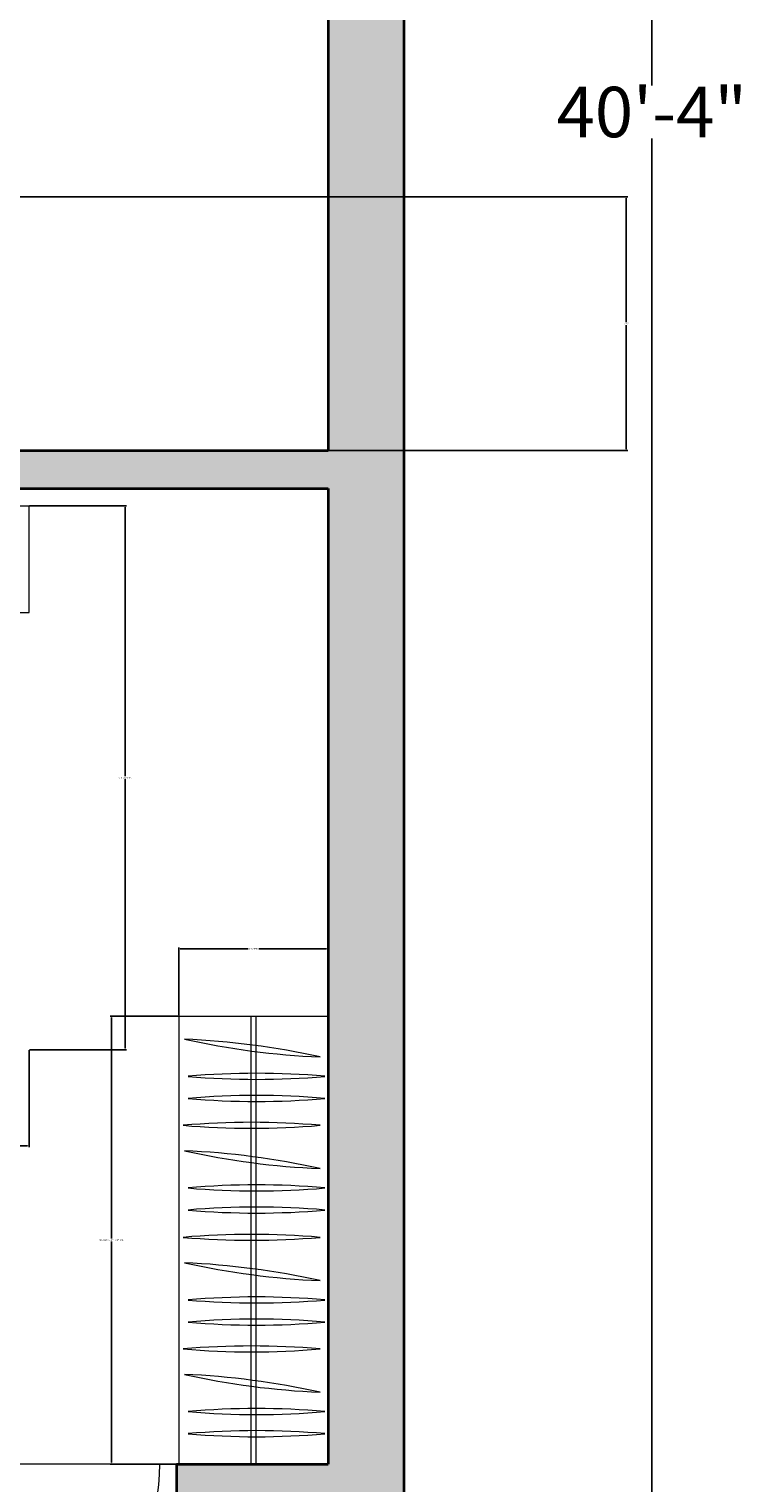
# Model space of a CAD drawing. Units: inches. Extents: x -5 to 366, y -496 to 54.
# Tile 7 of 10: x 280 to 366, y -378 to -205. Entities that reach past the tile are written whole.
import ezdxf

# ---------------------------------------------------------------- set-up
doc = ezdxf.new("R2010")
doc.units = ezdxf.units.IN
doc.header["$MEASUREMENT"] = 0
for name, color, linetype, lineweight in [('A-ANNO-DIMS', 2, 'Continuous', 18), ('A-DOOR', 3, 'Continuous', 18), ('A-FLOR-CASE', 7, 'Continuous', 25), ('A-FURN', 8, 'Continuous', 18), ('A-WALL', 7, 'Continuous', 35), ('A-WALL-PATT', 252, 'Continuous', 13)]:
    doc.layers.add(name, color=color, linetype=linetype, lineweight=lineweight)
doc.styles.get("Standard").update_dxf_attribs({"font": 'arial.ttf'})
doc.dimstyles.get("Standard").update_dxf_attribs({"dimtxt": 0.18, "dimasz": 0.18, "dimexe": 0.18, "dimexo": 0.0625, "dimgap": 0.09, "dimtad": 0, "dimtih": 1, "dimtoh": 1, "dimdec": 0, "dimzin": 0, "dimdsep": 46, "dimlunit": 3, "dimtxsty": 'Standard', "dimcen": 0.09, "dimadec": 0, "dimazin": 0, "dimtfac": 1, "dimtdec": 0, "dimtofl": 0, "dimtmove": 0, "dimatfit": 3, "dimfxl": 1, "dimtolj": 1, "dimtzin": 0, "dimarcsym": 0})

# ---------------------------------------------------------------- blocks, each defined once
blk = doc.blocks.new('*D3')
at = {"layer": 'A-ANNO-DIMS', "color": 0, "lineweight": -2, "transparency": 16777216}
for p, q in [((325, 26.52), (354.61, 26.52)), ((354.43, 26.34), (354.43, -212.08)), ((354.43, -456.8), (354.43, -218.38)), ((325, -456.98), (354.61, -456.98))]:
    blk.add_line(p, q, dxfattribs=at)
at = {"layer": 'A-ANNO-DIMS', "color": 0, "transparency": 16777216}
for points in [[(354.4, 26.34), (354.46, 26.34), (354.43, 26.52)], [(354.4, -456.8), (354.46, -456.8), (354.43, -456.98)]]:
    blk.add_solid(points, dxfattribs=at)
at = {"layer": 'Defpoints', "color": 0, "transparency": 16777216}
for p in [(324.93, 26.52), (324.93, -456.98), (354.43, -456.98)]:
    blk.add_point(p, dxfattribs=at)
at = {"layer": 'A-ANNO-DIMS', "color": 0, "transparency": 16777216, "insert": (354.43, -215.23), "char_height": 6, "attachment_point": 5}
blk.add_mtext('\\A1;40\'-4"', dxfattribs=at)
blk = doc.blocks.new('DOOR-SWING-24IN')
for p, q in [((-1, 0), (-1, 24)), ((0, 0), (0, 24))]:
    blk.add_line(p, q)
blk.add_arc((0, 0), 24, 90, 180)
blk = doc.blocks.new('BED-DOUBLE-WITH-NIGHTSTANDS')
for p, q in [((0, 64.67), (76.05, 64.67)), ((15.21, 64.67), (15.21, 43.8)), ((7.61, 53.37), (7.61, 63.31)), ((60.84, 63.7), (15.21, 63.7)), ((68.45, 53.37), (68.45, 63.31)), ((12.58, 58.34), (2.64, 58.34)), ((63.48, 58.34), (73.42, 58.34)), ((15.21, 52.66), (60.84, 52.66)), ((25.78, 50.4), (34.07, 52.66)), ((36.11, 52.66), (31.94, 46.86)), ((20.23, 48.39), (25.78, 50.4)), ((60.61, 48.72), (33, 48.33)), ((60.64, 49.5), (33.56, 49.12)), ((17.3, 46.24), (20.23, 48.39)), ((31.94, 46.86), (30.24, 42.39)), ((14.53, 43.01), (17.3, 46.24)), ((60.58, 45.54), (31.39, 45.42)), ((60.57, 46.32), (31.69, 46.21)), ((15.15, 42.39), (14.53, 43.01)), ((18.23, 42.7), (15.15, 42.39)), ((22.08, 42.39), (18.23, 42.7)), ((25.47, 41.93), (22.08, 42.39)), ((27.47, 41.01), (25.47, 41.93)), ((30.24, 42.39), (29.94, 40.39)), ((29.94, 40.39), (27.47, 41.01)), ((10.04, 27.39), (14.34, 27.39)), ((10.04, 0), (10.04, 27.39)), ((14.34, 26.51), (10.92, 26.51)), ((10.92, 26.51), (10.92, 0.88)), ((64.6, 26.51), (61.25, 26.51)), ((61.27, 27.39), (65.49, 27.39)), ((64.6, 0.88), (64.6, 26.51)), ((65.49, 27.39), (65.49, 0)), ((61.19, 22.65), (14.34, 22.65)), ((61.26, 21.7), (14.34, 21.7)), ((53.47, 14.23), (22.59, 14.23)), ((18.42, 8.59), (18.25, 9.45)), ((23.73, 8.59), (23.9, 9.45)), ((51.79, 8.59), (51.63, 9.45)), ((57.11, 8.59), (57.28, 9.45)), ((10.92, 0.88), (64.6, 0.88)), ((65.49, 0), (10.04, 0))]:
    blk.add_line(p, q)
for points in [[(15.21, 52), (0, 52), (0, 64.67)], [(60.84, 64.67), (60.84, 52), (76.05, 52), (76.05, 64.67)], [(7.61, 58.34), (8.49, 59.87)], [(68.45, 58.34), (67.56, 59.87)], [(7.61, 58.34), (8.49, 56.8)], [(68.45, 58.34), (67.56, 56.8)]]:
    blk.add_lwpolyline(points)
for points in [[(19.58, 62.78, 0.074897), (19.67, 57.81, -0.472817)], [(37.67, 57.53, 0.14099), (37.82, 62.6, 0.235245)], [(40.92, 57.53, -0.14099), (40.77, 62.6, -0.235245)], [(56.48, 62.78, -0.074897), (56.38, 57.81, 0.472817)], [(14.37, 36.04, 0.001242), (14.34, 21.61, -0.127202), (12.81, 14.42)], [(61.17, 23.25, 0.056112), (61.72, 19.07, 0.095341), (62.79, 15.03)]]:
    blk.add_lwpolyline(points, format="xyb")
for centre, radius in [((7.61, 58.34), 3.55), ((68.45, 58.34), 3.55), ((7.61, 58.34), 1.77), ((68.45, 58.34), 1.77), ((22.81, 5.83), 0.194), ((52.72, 5.83), 0.194), ((21.54, 3.79), 0.194), ((53.98, 3.79), 0.194)]:
    blk.add_circle(centre, radius)
for centre, radius, start, end in [((61.5, 786.54), 724.98, 266.68521, 267.14978), ((30, 35.26), 27.58, 82.2196, 99.497), ((35.83, 49.2), 13.55, 81.5249, 103.96), ((41.81, 58.99), 3.76, 63.3437, 106.1026), ((47.45, 49.47), 13.37, 76.3427, 101.1841), ((14.56, 786.54), 724.98, 272.85022, 273.31479), ((29.27, 55.82), 9.8, 155.1316, 191.7583), ((46.79, 55.82), 9.8, 348.2417, 24.8684), ((28.71, 54.99), 9.32, 354.0129, 15.8293), ((49.88, 54.99), 9.32, 164.1707, 185.9871), ((22.29, 63.67), 10.19, 255.1039, 281.0369), ((27.66, 70.91), 17.68, 258.0397, 289.2615), ((34.82, 67.05), 13.41, 259.8617, 283.6238), ((42.32, 57.67), 4.03, 245.0183, 288.5407), ((49.36, 62.92), 9.68, 243.8761, 286.1746), ((53.76, 63.67), 10.19, 258.9631, 284.8961), ((197.18, 43.36), 136.65, 176.1, 180.9282), ((-55.2, 41.12), 69.76, 355.8294, 1.553), ((15.83, 69.94), 28.7, 267.4519, 281.3392), ((22.69, 35.73), 6.19, 66.2616, 101.3392), ((35.22, 69.13), 29.49, 250.1194, 259.3383), ((29.76, 40.33), 0.184, 268.8623, 19.7536), ((238.78, 38.39), 178.26, 179.1145, 184.8735), ((13.51, 14.47), 0.702, 183.98, 297.3412), ((21.68, -64.93), 79.17, 89.3433, 95.6887), ((13.22, 8.88), 5.76, 33.6671, 63.2997), ((20.93, 12.3), 2.93, 145.785, 184.7304), ((15.33, 13.67), 3.15, 328.8218, 9.1554), ((19.23, 13.39), 0.916, 120.0293, 142.325), ((17.77, 12.85), 2.42, 289.2822, 29.1751), ((18.84, 13.57), 1.14, 311.5653, 23.8354), ((19.23, 13.39), 0.916, 44.4517, 63.558), ((24.38, 12.85), 2.42, 150.8249, 250.7178), ((23.31, 13.57), 1.14, 156.1646, 228.4347), ((22.92, 13.39), 0.916, 113.229, 135.5483), ((22.92, 13.39), 0.916, 37.675, 66.7144), ((21.22, 12.3), 2.93, 355.2696, 34.215), ((26.82, 13.67), 3.15, 169.7133, 211.1782), ((28.93, 8.88), 5.76, 111.4941, 146.3329), ((46.59, 8.88), 5.76, 33.6671, 68.5059), ((54.31, 12.3), 2.93, 145.785, 184.7304), ((48.7, 13.67), 3.15, 328.8218, 10.2867), ((52.61, 13.39), 0.916, 113.2856, 142.325), ((51.15, 12.85), 2.42, 289.2822, 29.1751), ((52.61, 13.39), 0.916, 44.4517, 66.7144), ((52.22, 13.57), 1.14, 311.5653, 23.8354), ((55.8, -59.74), 74, 85.2402, 91.8035), ((57.76, 12.85), 2.42, 150.8249, 250.7178), ((56.68, 13.57), 1.14, 156.1646, 228.4347), ((56.3, 13.39), 0.916, 106.6343, 135.5483), ((56.3, 13.39), 0.916, 37.675, 72.5814), ((54.6, 12.3), 2.93, 355.2696, 34.215), ((60.2, 13.67), 3.15, 169.249, 211.1782), ((62.31, 8.88), 5.76, 113.6453, 146.3329), ((62.21, 14.65), 0.693, 246.5219, 33.8264), ((16.57, 11.64), 1.28, 84.4856, 181.0538), ((16.17, 10.69), 2.29, 355.2933, 76.921), ((20.63, 11.55), 1.56, 131.5653, 195.1471), ((17.4, 12.41), 2.19, 7.436, 29.9149), ((21.52, 11.55), 1.56, 344.8529, 48.4347), ((24.75, 12.41), 2.19, 150.0851, 172.564), ((25.97, 10.69), 2.29, 103.079, 184.7067), ((25.58, 11.64), 1.28, 358.9462, 95.5144), ((49.95, 11.64), 1.28, 84.4856, 181.0538), ((49.55, 10.69), 2.29, 355.2933, 76.921), ((54.01, 11.55), 1.56, 131.5653, 195.1471), ((50.78, 12.41), 2.19, 7.436, 29.9149), ((54.89, 11.55), 1.56, 344.8529, 48.4347), ((58.13, 12.41), 2.19, 150.0851, 172.564), ((59.35, 10.69), 2.29, 103.079, 184.7067), ((58.96, 11.64), 1.28, 358.9462, 95.5144), ((17.09, 11.46), 1.82, 174.9449, 262.8857), ((17.81, 12.15), 1.76, 201.5819, 291.4221), ((16.78, 11.86), 2.21, 272.3591, 324.0401), ((14.38, 10.75), 4.08, 326.2883, 356.5076), ((17.47, 10.23), 1.89, 299.9085, 73.1337), ((20.93, 12.3), 2.93, 212.7011, 216.3445), ((18.67, 11.02), 0.472, 257.3041, 15.1471), ((21.29, 10.31), 0.147, 102.7051, 280.4384), ((21.28, 10.4), 0.238, 280.4384, 100.4136), ((24.67, 10.23), 1.89, 106.8663, 240.0915), ((23.48, 11.02), 0.472, 164.8529, 282.6959), ((21.22, 12.3), 2.93, 323.6555, 327.2989), ((25.37, 11.86), 2.21, 215.9599, 267.6409), ((24.34, 12.15), 1.76, 248.5779, 338.4181), ((27.77, 10.75), 4.08, 183.4924, 213.7117), ((25.05, 11.46), 1.82, 277.1143, 5.0551), ((50.47, 11.46), 1.82, 174.9449, 262.8857), ((51.19, 12.15), 1.76, 201.5819, 291.4221), ((50.16, 11.86), 2.21, 272.3591, 324.0401), ((47.76, 10.75), 4.08, 326.2883, 356.5076), ((50.85, 10.23), 1.89, 299.9085, 73.1337), ((54.31, 12.3), 2.93, 212.7011, 216.3445), ((52.05, 11.02), 0.472, 257.3041, 15.1471), ((54.25, 10.4), 0.238, 79.5864, 259.5616), ((54.23, 10.31), 0.147, 259.5616, 77.2949), ((58.05, 10.23), 1.89, 106.8663, 240.0915), ((56.86, 11.02), 0.472, 164.8529, 282.6959), ((54.6, 12.3), 2.93, 323.6555, 327.2989), ((58.75, 11.86), 2.21, 215.9599, 267.6409), ((57.72, 12.15), 1.76, 248.5779, 338.4181), ((61.15, 10.75), 4.08, 183.4924, 213.7117), ((58.43, 11.46), 1.82, 277.1143, 5.0551), ((16.68, 8.53), 1.14, 80.264, 250.8688), ((14.41, 11.04), 3.59, 301.2614, 341.7045), ((20.64, 8.49), 0.155, 55.7657, 157.4417), ((26.56, 6.48), 6.3, 153.0032, 159.8941), ((20.89, 8.63), 0.155, 84.3784, 186.0543), ((20.74, 9.25), 0.637, 269.1859, 301.164), ((20.93, 8.93), 0.365, 237.5332, 323.4768), ((20.57, 9.97), 1.22, 285.5129, 293.6099), ((21.37, 8.59), 0.399, 87.3579, 140.4944), ((20.45, 9.74), 1.2, 301.164, 321.5612), ((19.47, 9.95), 2.14, 324.6898, 333.4936), ((27.73, 11.04), 3.59, 198.2955, 238.7386), ((25.47, 8.53), 1.14, 289.1312, 99.736), ((38.62, -0.46), 9.93, 94.4623, 172.255), ((38.66, 8.7), 1.1, 137.7873, 219.1145), ((37.41, 8.74), 0.829, 298.5391, 58.3627), ((38.64, 9.21), 0.823, 63.0274, 163.8037), ((37.8, 11.14), 1.7, 271.4585, 315.3727), ((38.49, 8.01), 1.57, 45.5411, 114.3101), ((39.93, 16.07), 6.95, 252.593, 267.2582), ((38.66, 9.41), 0.812, 177.7585, 283.852), ((40.22, 10.26), 2.51, 198.9159, 238.011), ((39.57, 8.01), 1.57, 65.6899, 134.4589), ((38.14, 16.07), 6.95, 272.7418, 287.407), ((38.83, 8.73), 0.107, 283.852, 219.9245), ((39.42, 9.21), 0.823, 16.1963, 116.9726), ((40.26, 11.14), 1.7, 224.6273, 268.5415), ((39.22, 8.77), 0.0647, 320.1909, 256.0209), ((37.84, 10.26), 2.51, 301.989, 341.0841), ((39.4, 9.41), 0.812, 256.148, 2.2415), ((40.65, 8.74), 0.829, 121.6373, 241.4609), ((39.4, 8.7), 1.1, 320.8855, 42.2127), ((39.12, 1.83), 7.69, 352.8636, 81.8197), ((50.06, 8.53), 1.14, 80.264, 250.8688), ((47.79, 11.04), 3.59, 301.2614, 341.7045), ((55.08, 9.74), 1.2, 218.4388, 238.836), ((54.15, 8.59), 0.399, 39.5056, 92.6421), ((56.06, 9.95), 2.14, 206.5064, 215.3102), ((54.6, 8.93), 0.365, 216.5232, 302.4668), ((54.95, 9.97), 1.22, 246.3901, 254.4871), ((54.79, 9.25), 0.637, 238.836, 270.8141), ((48.96, 6.48), 6.3, 20.1059, 26.9968), ((54.64, 8.63), 0.155, 353.9457, 95.6216), ((54.88, 8.49), 0.155, 22.5583, 124.2343), ((61.11, 11.04), 3.59, 198.2955, 238.7386), ((58.85, 8.53), 1.14, 289.1312, 99.736), ((15.71, 6.95), 0.823, 92.9516, 193.728), ((14.03, 8.2), 1.7, 301.3827, 345.2969), ((16.18, 5.84), 1.57, 75.4653, 144.2343), ((13.4, 13.54), 6.95, 282.5173, 297.1824), ((16.44, 7.29), 0.7, 63.9755, 143.2681), ((16.4, 8.87), 1.43, 265.969, 344.3045), ((17.94, 6.98), 1.52, 96.1662, 141.5825), ((19.32, 7.28), 0.323, 101.5637, 142.6358), ((19.06, 6.98), 0.194, 273.2768, 86.7232), ((19.28, 7.17), 0.185, 91.1081, 181.8675), ((19.48, 6.8), 0.4, 80.3487, 133.6538), ((19.06, 7.54), 0.466, 288.7263, 352.5032), ((19.4, 6.38), 0.634, 83.0852, 105.7171), ((19.38, 7.52), 0.15, 345.2356, 144.9248), ((19.52, 7.03), 0.167, 317.6792, 80.3487), ((20.45, 8.04), 0.399, 101.3256, 154.4621), ((19.88, 9.4), 1.2, 280.2588, 300.656), ((20.15, 10.36), 2.14, 268.3264, 277.1302), ((26.56, 6.48), 6.3, 163.5842, 183.8277), ((19.62, 9.39), 1.22, 308.2101, 316.3071), ((20.37, 8.59), 0.365, 278.3432, 4.2869), ((20.17, 8.91), 0.637, 300.656, 332.6341), ((24.21, 6.98), 1.52, 38.4175, 83.8338), ((25.74, 8.87), 1.43, 195.6955, 274.031), ((25.71, 7.29), 0.7, 36.7319, 116.0245), ((25.96, 5.84), 1.57, 35.7657, 104.5347), ((28.74, 13.54), 6.95, 242.8176, 257.4827), ((26.44, 6.95), 0.823, 346.272, 87.0484), ((28.12, 8.2), 1.7, 194.7031, 238.6173), ((38.96, 8.23), 0.123, 238.011, 71.5592), ((38.98, 8.29), 0.0599, 71.5592, 188.0167), ((39.1, 8.23), 0.123, 108.4408, 301.989), ((39.08, 8.29), 0.0599, 351.9833, 108.4408), ((49.09, 6.95), 0.823, 92.9516, 193.728), ((47.41, 8.2), 1.7, 301.3827, 345.2969), ((49.56, 5.84), 1.57, 75.4653, 144.2343), ((46.78, 13.54), 6.95, 282.5173, 297.1824), ((49.82, 7.29), 0.7, 63.9755, 143.2681), ((49.78, 8.87), 1.43, 265.969, 344.3045), ((51.32, 6.98), 1.52, 96.1662, 141.5825), ((55.16, 8.59), 0.365, 175.7131, 261.6568), ((55.36, 8.91), 0.637, 207.3659, 239.344), ((48.96, 6.48), 6.3, 356.1723, 16.4158), ((55.91, 9.39), 1.22, 223.6929, 231.7899), ((55.65, 9.4), 1.2, 239.344, 259.7412), ((55.37, 10.36), 2.14, 262.8698, 271.6736), ((55.07, 8.04), 0.399, 25.5379, 78.6744), ((56.01, 7.03), 0.167, 99.6513, 222.3208), ((56.05, 6.8), 0.4, 46.3462, 99.6513), ((56.15, 7.52), 0.15, 35.0752, 194.7644), ((56.46, 7.54), 0.466, 187.4968, 251.2737), ((56.12, 6.38), 0.634, 74.2829, 96.9148), ((56.25, 7.17), 0.185, 358.1325, 88.8919), ((56.2, 7.28), 0.323, 37.3642, 78.4363), ((56.47, 6.98), 0.194, 93.2768, 266.7232), ((59.12, 8.87), 1.43, 195.6955, 274.031), ((57.59, 6.98), 1.52, 38.4175, 83.8338), ((59.08, 7.29), 0.7, 36.7319, 116.0245), ((59.34, 5.84), 1.57, 35.7657, 104.5347), ((62.12, 13.54), 6.95, 242.8176, 257.4827), ((61.5, 8.2), 1.7, 194.7031, 238.6173), ((59.82, 6.95), 0.823, 346.272, 87.0484), ((3.53, -0.46), 9.93, 7.745, 41.8856), ((20.52, -1.44), 9.93, 124.3865, 158.5908), ((15.99, 6.52), 1.1, 167.7115, 249.0387), ((14.89, 5.93), 0.829, 328.4633, 88.2869), ((16.56, 8.65), 2.51, 228.8402, 267.9352), ((15.63, 7.13), 0.812, 207.6827, 313.7762), ((16.12, 6.62), 0.107, 313.7762, 249.7183), ((16.46, 6.32), 0.0599, 101.4834, 217.9409), ((16.48, 6.26), 0.123, 267.9352, 101.4834), ((19.32, 6.63), 0.32, 217.7621, 259.0403), ((19.66, 7.05), 0.588, 203.4276, 227.6104), ((19.41, 7.13), 0.317, 229.7889, 317.6792), ((19.05, 6.46), 0.45, 355.053, 68.3618), ((19.35, 6.43), 0.149, 232.4737, 355.053), ((15.01, 1.12), 7.22, 43.1541, 52.0459), ((20, 5.48), 0.399, 101.3256, 154.4621), ((19.42, 6.84), 1.2, 280.2588, 300.656), ((19.7, 7.8), 2.14, 268.3264, 277.1302), ((19.17, 6.83), 1.22, 308.2101, 316.3071), ((19.91, 6.03), 0.365, 278.3432, 4.2869), ((19.71, 6.35), 0.637, 300.656, 332.6341), ((20.19, 5.93), 0.155, 55.7657, 157.4417), ((23.43, 6.32), 3.16, 184.756, 209.2041), ((27.97, 13.04), 10.39, 222.2412, 232.1744), ((23.75, 2.13), 3.79, 120.544, 139.818), ((21.33, 6.12), 0.883, 304.5369, 16.3699), ((21.8, 5.92), 0.537, 272.8499, 356.1226), ((21.42, 5.72), 0.52, 321.7607, 7.9252), ((21.53, 4.97), 0.52, 8.7227, 54.8872), ((21.56, 4.55), 0.883, 0.278, 72.111), ((22.55, 5.87), 0.625, 127.3105, 187.9252), ((21.95, 4.88), 0.537, 20.5253, 88.5375), ((21.7, 5.94), 0.641, 355.0106, 41.658), ((22.4, 5.47), 0.192, 148.0499, 225.6268), ((23.75, 2.13), 3.79, 113.0501, 113.8477), ((22.76, 5.25), 0.611, 104.7558, 148.0499), ((22.42, 5.69), 0.382, 247.4086, 351.4386), ((22.6, 6.1), 0.264, 126.1046, 271.4281), ((22.57, 6.17), 0.19, 353.7526, 131.7054), ((22.52, 5.67), 0.128, 262.906, 7.132), ((22.39, 5.95), 0.267, 0.0645, 61.1507), ((22.45, 6.18), 0.305, 311.8413, 355.7877), ((23.07, 5.47), 0.32, 151.2196, 259.0403), ((23.08, 6.13), 0.323, 101.5637, 176.365), ((23.04, 6.02), 0.185, 91.1081, 181.8675), ((23.42, 5.9), 0.588, 203.4276, 227.6104), ((23.23, 5.64), 0.4, 80.3487, 133.6538), ((23.16, 5.98), 0.317, 229.7889, 317.6792), ((22.82, 6.39), 0.466, 288.7263, 352.5032), ((22.8, 5.3), 0.45, 355.053, 68.3618), ((23.16, 5.23), 0.634, 83.0852, 105.7171), ((23.14, 6.36), 0.15, 345.2356, 144.9248), ((23.1, 5.28), 0.149, 232.4737, 355.053), ((23.27, 5.87), 0.167, 317.6792, 80.3487), ((23.75, 2.13), 3.79, 87.1071, 94.7585), ((25.67, 6.26), 0.123, 78.5166, 272.0648), ((25.58, 8.65), 2.51, 272.0648, 311.1598), ((25.68, 6.32), 0.0599, 322.0591, 78.5166), ((26.52, 7.13), 0.812, 226.2238, 332.3173), ((26.04, 6.66), 0.0647, 290.2667, 226.2271), ((27.26, 5.93), 0.829, 91.7131, 211.5367), ((26.16, 6.52), 1.1, 290.9613, 12.2885), ((21.63, -1.44), 9.93, 21.4092, 55.6135), ((53.9, -1.44), 9.93, 124.3865, 158.5908), ((49.36, 6.52), 1.1, 167.7115, 249.0387), ((49.01, 7.13), 0.812, 207.6827, 313.7762), ((49.94, 8.65), 2.51, 228.8402, 267.9352), ((48.26, 5.93), 0.829, 328.4633, 88.2869), ((49.5, 6.62), 0.107, 313.7762, 249.7183), ((49.84, 6.32), 0.0599, 101.4834, 217.9409), ((49.86, 6.26), 0.123, 267.9352, 101.4834), ((51.78, 2.13), 3.79, 85.2415, 92.8929), ((52.25, 5.87), 0.167, 99.6513, 222.3208), ((52.37, 5.98), 0.317, 222.3208, 310.2111), ((52.29, 5.64), 0.4, 46.3462, 99.6513), ((52.39, 6.36), 0.15, 35.0752, 194.7644), ((52.71, 6.39), 0.466, 187.4968, 251.2737), ((52.72, 5.3), 0.45, 111.6382, 184.947), ((52.42, 5.28), 0.149, 184.947, 307.5263), ((52.37, 5.23), 0.634, 74.2829, 96.9148), ((52.49, 6.02), 0.185, 358.1325, 88.8919), ((52.11, 5.9), 0.588, 312.3896, 336.5724), ((52.45, 6.13), 0.323, 3.635, 78.4363), ((52.45, 5.47), 0.32, 280.9597, 28.7804), ((53.11, 5.69), 0.382, 188.5614, 292.5914), ((52.96, 6.17), 0.19, 48.2946, 186.2474), ((53.07, 6.18), 0.305, 184.2123, 228.1587), ((53.14, 5.95), 0.267, 118.8493, 179.9355), ((53, 5.67), 0.128, 172.868, 277.094), ((52.93, 6.1), 0.264, 268.5719, 53.8954), ((52.77, 5.25), 0.611, 31.9501, 75.2442), ((53.57, 4.88), 0.537, 91.4625, 159.4747), ((53.97, 4.55), 0.883, 107.889, 179.722), ((53.83, 5.94), 0.641, 138.342, 184.9894), ((53.73, 5.92), 0.537, 183.8774, 267.1501), ((51.78, 2.13), 3.79, 66.1523, 66.9499), ((53.12, 5.47), 0.192, 314.3732, 31.9501), ((54.2, 6.12), 0.883, 163.6301, 235.4631), ((52.97, 5.87), 0.625, 352.0748, 52.6895), ((54, 4.97), 0.52, 125.1128, 171.2773), ((54.11, 5.72), 0.52, 172.0748, 218.2393), ((51.78, 2.13), 3.79, 40.182, 59.456), ((47.55, 13.04), 10.39, 307.8256, 317.7588), ((52.1, 6.32), 3.16, 330.7959, 355.244), ((60.52, 1.12), 7.22, 127.9541, 136.8459), ((55.33, 5.93), 0.155, 22.5583, 124.2343), ((55.61, 6.03), 0.365, 175.7131, 261.6568), ((55.81, 6.35), 0.637, 207.3659, 239.344), ((56.36, 6.83), 1.22, 223.6929, 231.7899), ((56.1, 6.84), 1.2, 239.344, 259.7412), ((55.82, 7.8), 2.14, 262.8698, 271.6736), ((55.53, 5.48), 0.399, 25.5379, 78.6744), ((56.12, 7.13), 0.317, 222.3208, 310.2111), ((56.48, 6.46), 0.45, 111.6382, 184.947), ((56.18, 6.43), 0.149, 184.947, 307.5263), ((55.86, 7.05), 0.588, 312.3896, 336.5724), ((56.21, 6.63), 0.32, 280.9597, 322.2379), ((59.05, 6.26), 0.123, 78.5166, 272.0648), ((58.96, 8.65), 2.51, 272.0648, 311.1598), ((59.06, 6.32), 0.0599, 322.0591, 78.5166), ((59.9, 7.13), 0.812, 226.2238, 332.3173), ((59.42, 6.66), 0.0647, 290.2667, 226.2271), ((60.64, 5.93), 0.829, 91.7131, 211.5367), ((59.54, 6.52), 1.1, 290.9613, 12.2885), ((55.01, -1.44), 9.93, 21.4092, 55.6135), ((72, -0.46), 9.93, 138.1144, 172.255), ((20.13, 4.78), 0.216, 146.8636, 236.9021), ((23.18, 9.55), 5.66, 235.1882, 238.8844), ((20.5, 5.1), 0.585, 199.4799, 267.6828), ((20.44, 4.87), 0.504, 212.8155, 277.3992), ((20.15, 4.54), 0.585, 266.9701, 338.2913), ((17.06, 8.72), 5.66, 302.6784, 306.3746), ((20.29, 4.07), 0.216, 214.3538, 304.3923), ((20.37, 4.89), 0.224, 238.8844, 314.2646), ((20.33, 4.39), 0.504, 280.3057, 17.1958), ((20.28, 4.34), 0.224, 306.3746, 21.7548), ((20.65, 4.49), 0.169, 19.3605, 201.7548), ((20.65, 4.61), 0.169, 311.8703, 134.2646), ((23.82, 3.07), 3.37, 153.7819, 158.2913), ((21.14, 5.38), 0.883, 247.2305, 319.0635), ((20.85, 5.08), 0.52, 264.4544, 310.6188), ((23.43, 6.32), 3.16, 214.0033, 222.4917), ((21.23, 4.87), 0.537, 218.3208, 298.8162), ((21.14, 3.43), 0.192, 148.0499, 225.6268), ((21.49, 3.21), 0.611, 104.7558, 148.0499), ((21.15, 3.64), 0.382, 247.4086, 351.4386), ((21.33, 4.06), 0.264, 126.1046, 271.4281), ((21.3, 4.13), 0.19, 353.7526, 131.7054), ((21.59, 4.21), 0.625, 70.0041, 130.6188), ((21.26, 3.63), 0.128, 262.906, 7.132), ((21.12, 3.91), 0.267, 0.0645, 61.1507), ((21.18, 4.13), 0.305, 311.8413, 355.7877), ((21.19, 4.97), 0.641, 297.7043, 344.3516), ((21.81, 4.09), 0.323, 101.5637, 176.365), ((21.81, 3.43), 0.32, 151.2196, 259.0403), ((21.77, 3.98), 0.185, 91.1081, 181.8675), ((22.15, 3.86), 0.588, 203.4276, 227.6104), ((21.97, 3.6), 0.4, 80.3487, 133.6538), ((21.89, 3.93), 0.317, 229.7889, 317.6792), ((21.55, 4.35), 0.466, 288.7263, 352.5032), ((21.54, 3.26), 0.45, 355.053, 68.3618), ((21.89, 3.19), 0.634, 83.0852, 105.7171), ((21.87, 4.32), 0.15, 345.2356, 144.9248), ((22, 3.83), 0.167, 317.6792, 80.3487), ((22.66, 5.14), 0.625, 188.7227, 249.3375), ((21.86, 4.83), 0.641, 334.9899, 21.6373), ((37.86, -5.78), 9.93, 94.4623, 117.4146), ((37.9, 3.38), 1.1, 137.7873, 219.1145), ((36.65, 3.42), 0.829, 298.5391, 58.3627), ((37.88, 3.89), 0.823, 63.0274, 163.8037), ((37.04, 5.82), 1.7, 271.4585, 315.3727), ((37.73, 2.69), 1.57, 45.5411, 114.3101), ((39.46, 4.94), 2.51, 198.9159, 238.011), ((39.17, 10.75), 6.95, 252.593, 267.2582), ((37.9, 4.09), 0.812, 177.7585, 283.852), ((38.07, 3.41), 0.107, 283.852, 219.9245), ((40.33, 2.69), 1.57, 65.6899, 134.4589), ((38.9, 10.75), 6.95, 272.7418, 287.407), ((40.18, 3.89), 0.823, 16.1963, 116.9726), ((41.02, 5.82), 1.7, 224.6273, 268.5415), ((39.98, 3.45), 0.0647, 320.1909, 256.0209), ((38.6, 4.94), 2.51, 301.989, 341.0841), ((40.16, 4.09), 0.812, 256.148, 2.2415), ((41.41, 3.42), 0.829, 121.6373, 241.4609), ((40.16, 3.38), 1.1, 320.8855, 42.2127), ((40.2, -5.78), 9.93, 62.5854, 85.5377), ((53.67, 4.83), 0.641, 158.3627, 205.0101), ((52.87, 5.14), 0.625, 290.6625, 351.2773), ((53.52, 3.83), 0.167, 99.6513, 222.3208), ((53.63, 3.93), 0.317, 222.3208, 310.2111), ((53.56, 3.6), 0.4, 46.3462, 99.6513), ((53.66, 4.32), 0.15, 35.0752, 194.7644), ((53.97, 4.35), 0.466, 187.4968, 251.2737), ((53.99, 3.26), 0.45, 111.6382, 184.947), ((53.64, 3.19), 0.634, 74.2829, 96.9148), ((53.93, 4.21), 0.625, 49.3812, 109.9959), ((54.39, 5.38), 0.883, 220.9365, 292.7695), ((54.34, 4.97), 0.641, 195.6484, 242.2957), ((53.76, 3.98), 0.185, 358.1325, 88.8919), ((53.37, 3.86), 0.588, 312.3896, 336.5724), ((53.72, 4.09), 0.323, 3.635, 78.4363), ((53.72, 3.43), 0.32, 280.9597, 28.7804), ((54.38, 3.64), 0.382, 188.5614, 292.5914), ((54.3, 4.87), 0.537, 241.1838, 321.6792), ((54.23, 4.13), 0.19, 48.2946, 186.2474), ((54.34, 4.13), 0.305, 184.2123, 228.1587), ((54.4, 3.91), 0.267, 118.8493, 179.9355), ((54.27, 3.63), 0.128, 172.868, 277.094), ((54.2, 4.06), 0.264, 268.5719, 53.8954), ((54.03, 3.21), 0.611, 31.9501, 75.2442), ((54.68, 5.08), 0.52, 229.3812, 275.5456), ((52.1, 6.32), 3.16, 317.5083, 325.9967), ((54.39, 3.43), 0.192, 314.3732, 31.9501), ((55.2, 4.39), 0.504, 162.8042, 259.6943), ((54.88, 4.61), 0.169, 45.7354, 228.1297), ((54.88, 4.49), 0.169, 338.2452, 160.6395), ((51.7, 3.07), 3.37, 21.7087, 26.2181), ((55.38, 4.54), 0.585, 201.7087, 273.0299), ((55.15, 4.89), 0.224, 225.7354, 301.1156), ((55.09, 4.87), 0.504, 262.6008, 327.1845), ((55.24, 4.34), 0.224, 158.2452, 233.6254), ((55.02, 5.1), 0.585, 272.3172, 340.5201), ((58.47, 8.72), 5.66, 233.6254, 237.3216), ((55.23, 4.07), 0.216, 235.6077, 325.6462), ((52.34, 9.55), 5.66, 301.1156, 304.8118), ((55.39, 4.78), 0.216, 303.0979, 33.1364), ((8.51, -1.79), 4.84, 33.4617, 60.1116), ((11.22, -0.67), 4.04, 22.5547, 48.9546), ((0.16, 1.5), 13.74, 357.4081, 3.6519), ((21.84, 3.24), 0.149, 232.4737, 355.053), ((30.93, -0.67), 4.04, 131.0454, 157.4453), ((41.99, 1.5), 13.74, 176.3481, 182.5919), ((33.64, -1.79), 4.84, 91.272, 146.5383), ((35.38, -2.69), 6.03, 107.8504, 143.6964), ((38.55, -4.39), 8.97, 124.0123, 144.053), ((38.2, 2.91), 0.123, 238.011, 71.5592), ((38.22, 2.97), 0.0599, 71.5592, 188.0167), ((39.86, 2.91), 0.123, 108.4408, 301.989), ((39.84, 2.97), 0.0599, 351.9833, 108.4408), ((40.11, 2.54), 4.45, 338.117, 6.6195), ((44.19, 1.3), 1.78, 346.3898, 79.0739), ((42.85, 1.54), 2.25, 342.8609, 41.9049), ((33.54, 1.5), 13.74, 357.4081, 3.6519), ((44.6, -0.67), 4.04, 22.5547, 48.9546), ((53.69, 3.24), 0.149, 184.947, 307.5263), ((64.31, -0.67), 4.04, 131.0454, 157.4453), ((75.37, 1.5), 13.74, 176.3481, 182.5919), ((67.02, -1.79), 4.84, 119.8884, 146.5383), ((6.77, -2.69), 6.03, 36.3036, 46.4814), ((35.08, -4.34), 5.46, 73.5431, 107.0202), ((37.25, -7.16), 8.08, 94.3787, 95.6357), ((41.5, -12.69), 14.43, 109.7217, 109.9028), ((42.98, -4.34), 5.46, 72.9798, 106.4569), ((40.82, -7.16), 8.08, 84.3643, 85.6213), ((36.56, -12.69), 14.43, 70.0972, 70.2783), ((68.76, -2.69), 6.03, 133.5186, 143.6964)]:
    blk.add_arc(centre, radius, start, end)
blk = doc.blocks.new('WARDROBE-HANGING')
for p, q in [((0, 53.26), (0, 0)), ((0, 53.26), (17.76, 53.26)), ((8.58, 53.26), (8.58, 0)), ((9.18, 53.26), (9.18, 0)), ((17.76, 53.26), (17.76, 0)), ((0, 0), (17.76, 0))]:
    blk.add_line(p, q)
for centre, start, end in [((20.87, 141.73), 257.508, 267.5023), ((-3.4, -42.81), 77.508, 87.5023), ((9.24, -46.96), 85.0028, 94.9972), ((9.24, 139.16), 265.0028, 274.9972), ((9.24, -49.59), 85.0028, 94.9972), ((9.24, 136.53), 265.0028, 274.9972), ((8.66, -52.79), 85.0028, 94.9972), ((8.66, 133.34), 265.0028, 274.9972), ((20.87, 128.46), 257.508, 267.5023), ((-3.4, -56.08), 77.508, 87.5023), ((9.24, -60.23), 85.0028, 94.9972), ((9.24, 125.89), 265.0028, 274.9972), ((9.24, -62.86), 85.0028, 94.9972), ((9.24, 123.26), 265.0028, 274.9972), ((8.66, -66.11), 85.0028, 94.9972), ((8.66, 120.02), 265.0028, 274.9972), ((-3.4, -69.4), 77.508, 87.5023), ((20.87, 115.14), 257.508, 267.5023), ((9.24, -73.55), 85.0028, 94.9972), ((9.24, 112.57), 265.0028, 274.9972), ((9.24, -76.18), 85.0028, 94.9972), ((9.24, 109.94), 265.0028, 274.9972), ((8.66, -79.38), 85.0028, 94.9972), ((8.66, 106.75), 265.0028, 274.9972), ((-3.4, -82.67), 77.508, 87.5023), ((20.87, 101.87), 257.508, 267.5023), ((9.24, -86.82), 85.0028, 94.9972), ((9.24, 99.3), 265.0028, 274.9972), ((9.24, -89.45), 85.0028, 94.9972), ((9.24, 96.67), 265.0028, 274.9972)]:
    blk.add_arc(centre, 93.42, start, end)
blk = doc.blocks.new('*D15')
at = {"layer": 'A-ANNO-DIMS', "color": 0, "lineweight": -2, "transparency": 16777216}
for p, q in [((204.33, -326.78), (204.33, -338.31)), ((280.38, -326.78), (280.38, -338.31)), ((204.51, -338.13), (240.37, -338.13)), ((280.2, -338.13), (244.34, -338.13))]:
    blk.add_line(p, q, dxfattribs=at)
at = {"layer": 'A-ANNO-DIMS', "color": 0, "transparency": 16777216}
for points in [[(204.51, -338.1), (204.51, -338.16), (204.33, -338.13)], [(280.2, -338.1), (280.2, -338.16), (280.38, -338.13)]]:
    blk.add_solid(points, dxfattribs=at)
at = {"layer": 'Defpoints', "color": 0, "transparency": 16777216}
for p in [(204.33, -326.72), (280.38, -326.72), (280.38, -338.13)]:
    blk.add_point(p, dxfattribs=at)
at = {"layer": 'A-ANNO-DIMS', "color": 0, "transparency": 16777216, "insert": (242.35, -338.13), "char_height": 0.18, "attachment_point": 5}
blk.add_mtext('\\A1;BED & NIGHTSTANDS 6\'-4" TYP.', dxfattribs=at)
blk = doc.blocks.new('*D16')
at = {"layer": 'A-ANNO-DIMS', "color": 0, "lineweight": -2, "transparency": 16777216}
for p, q in [((280.44, -262.04), (291.97, -262.04)), ((291.79, -262.22), (291.79, -294.2)), ((291.79, -326.54), (291.79, -294.56)), ((280.44, -326.72), (291.97, -326.72))]:
    blk.add_line(p, q, dxfattribs=at)
at = {"layer": 'A-ANNO-DIMS', "color": 0, "transparency": 16777216}
for points in [[(291.76, -262.22), (291.82, -262.22), (291.79, -262.04)], [(291.76, -326.54), (291.82, -326.54), (291.79, -326.72)]]:
    blk.add_solid(points, dxfattribs=at)
at = {"layer": 'Defpoints', "color": 0, "transparency": 16777216}
for p in [(280.38, -262.04), (291.79, -262.04), (280.38, -326.72)]:
    blk.add_point(p, dxfattribs=at)
at = {"layer": 'A-ANNO-DIMS', "color": 0, "transparency": 16777216, "insert": (291.79, -294.38), "char_height": 0.18, "attachment_point": 5}
blk.add_mtext('\\A1;5\'-4 1/2" TYP.', dxfattribs=at)
blk = doc.blocks.new('*D17')
at = {"layer": 'A-ANNO-DIMS', "color": 0, "lineweight": -2, "transparency": 16777216}
for p, q in [((298.12, -322.72), (290.01, -322.72)), ((290.19, -322.9), (290.19, -349.16)), ((290.19, -375.8), (290.19, -349.53)), ((298.12, -375.98), (290.01, -375.98))]:
    blk.add_line(p, q, dxfattribs=at)
at = {"layer": 'A-ANNO-DIMS', "color": 0, "transparency": 16777216}
for points in [[(290.16, -322.9), (290.22, -322.9), (290.19, -322.72)], [(290.16, -375.8), (290.22, -375.8), (290.19, -375.98)]]:
    blk.add_solid(points, dxfattribs=at)
at = {"layer": 'Defpoints', "color": 0, "transparency": 16777216}
for p in [(290.19, -322.72), (298.18, -322.72), (298.18, -375.98)]:
    blk.add_point(p, dxfattribs=at)
at = {"layer": 'A-ANNO-DIMS', "color": 0, "transparency": 16777216, "insert": (290.19, -349.35), "char_height": 0.18, "attachment_point": 5}
blk.add_mtext('\\A1;WARDROBE 4\'-5 1/2" TYP.', dxfattribs=at)
blk = doc.blocks.new('*D18')
at = {"layer": 'A-ANNO-DIMS', "color": 0, "lineweight": -2, "transparency": 16777216}
for p, q in [((298.18, -322.65), (298.18, -314.55)), ((315.93, -322.65), (315.93, -314.55)), ((298.36, -314.73), (306.43, -314.73)), ((315.75, -314.73), (307.69, -314.73))]:
    blk.add_line(p, q, dxfattribs=at)
at = {"layer": 'A-ANNO-DIMS', "color": 0, "transparency": 16777216}
for points in [[(298.36, -314.7), (298.36, -314.76), (298.18, -314.73)], [(315.75, -314.7), (315.75, -314.76), (315.93, -314.73)]]:
    blk.add_solid(points, dxfattribs=at)
at = {"layer": 'Defpoints', "color": 0, "transparency": 16777216}
for p in [(315.93, -314.73), (298.18, -322.72), (315.93, -322.72)]:
    blk.add_point(p, dxfattribs=at)
at = {"layer": 'A-ANNO-DIMS', "color": 0, "transparency": 16777216, "insert": (307.06, -314.73), "char_height": 0.18, "attachment_point": 5}
blk.add_mtext('\\A1;1\'-6" TYP.', dxfattribs=at)
blk = doc.blocks.new('*D31')
at = {"layer": 'A-ANNO-DIMS', "color": 0, "lineweight": -2, "transparency": 16777216}
for p, q in [((316, -225.3), (351.56, -225.3)), ((351.38, -225.48), (351.38, -240.21)), ((351.38, -255.3), (351.38, -240.57)), ((316, -255.48), (351.56, -255.48))]:
    blk.add_line(p, q, dxfattribs=at)
at = {"layer": 'A-ANNO-DIMS', "color": 0, "transparency": 16777216}
for points in [[(351.35, -225.48), (351.41, -225.48), (351.38, -225.3)], [(351.35, -255.3), (351.41, -255.3), (351.38, -255.48)]]:
    blk.add_solid(points, dxfattribs=at)
at = {"layer": 'Defpoints', "color": 0, "transparency": 16777216}
for p in [(315.93, -225.3), (315.93, -255.48), (351.38, -255.48)]:
    blk.add_point(p, dxfattribs=at)
at = {"layer": 'A-ANNO-DIMS', "color": 0, "transparency": 16777216, "insert": (351.38, -240.39), "char_height": 0.18, "attachment_point": 5}
blk.add_mtext('\\A1;2\'-6"', dxfattribs=at)

msp = doc.modelspace()

# ---------------------------------------------------------------- hatches: boundary and pattern name
at = {"layer": 'A-WALL-PATT'}
h = msp.add_hatch(color=256, dxfattribs=at)
h.dxf.hatch_style = 1
h.paths.add_polyline_path([(324.93, 26.52), (21.93, 26.52), (21.93, -456.98), (26.43, -456.98), (26.43, -331.98), (30.93, -331.98), (30.93, -322.98), (30.93, -106.98), (110.93, -106.98), (110.93, -104.73), (110.93, -102.48), (30.93, -102.48), (30.93, 17.52), (138.93, 17.52), (141.18, 17.52), (143.43, 17.52), (183.43, 17.52), (187.93, 17.52), (315.93, 17.52), (315.93, -102.48), (315.93, -106.98), (315.93, -255.48), (171.93, -255.48), (171.93, -155.84), (167.43, -155.84), (167.43, -291.98), (171.93, -291.98), (171.93, -259.98), (315.93, -259.98), (315.93, -375.98), (297.93, -375.98), (297.93, -380.48), (315.93, -380.48), (315.93, -452.48), (315.93, -456.98), (324.93, -456.98)])
h.paths.add_polyline_path([(143.43, -18.48), (143.43, -13.98), (138.93, -13.98), (138.93, -106.98), (187.93, -106.98), (187.93, -102.48), (143.43, -102.48)], flags=17)

# ---------------------------------------------------------------- linework, layer by layer
at = {"layer": 'A-DOOR'}
for q in [(271.93, -375.98), (297.93, -375.98)]:
    msp.add_line((295.93, -375.98), q, dxfattribs=at)
at = {"layer": 'A-FLOR-CASE'}
msp.add_line((171.93, -225.3), (315.93, -225.3), dxfattribs=at)
at = {"layer": 'A-WALL'}
for p, q in [((324.93, 26.52), (324.93, -456.98)), ((315.93, -106.98), (315.93, -255.48)), ((171.93, -255.48), (315.93, -255.48)), ((171.93, -259.98), (315.93, -259.98)), ((315.93, -259.98), (315.93, -375.98)), ((297.93, -375.98), (297.93, -380.48)), ((297.93, -375.98), (315.93, -375.98))]:
    msp.add_line(p, q, dxfattribs=at)

# ---------------------------------------------------------------- block references
at = {"layer": 'A-DOOR', "rotation": 180}
msp.add_blockref('DOOR-SWING-24IN', (271.93, -375.98), dxfattribs=at)
at = {"layer": 'A-FURN'}
for name, p in [('BED-DOUBLE-WITH-NIGHTSTANDS', (204.33, -326.72)), ('WARDROBE-HANGING', (298.18, -375.98))]:
    msp.add_blockref(name, p, dxfattribs=at)

# ---------------------------------------------------------------- dimensions: what is measured, and where the dimension line sits
at = {"layer": 'A-ANNO-DIMS'}
for base, p1, p2, override, picture, middle in [((354.42742117, -456.97937362), (324.93325287, 26.52062638), (324.93325287, -456.97937362), {"dimtxt": 6, "dimclrd": 0, "dimclre": 0, "dimclrt": 0}, '*D3', (354.42742117, -215.22937362)), ((351.38, -255.48), (315.93, -225.3), (315.93, -255.48), {"dimdec": 1, "dimlfac": 1, "dimrnd": 0, "dimzin": 1, "dimdsep": 46, "dimlunit": 4, "dimfrac": 2}, '*D31', (351.38, -240.39))]:
    dim = msp.add_linear_dim(base=base, p1=p1, p2=p2, angle=90, dimstyle='Standard', override=override, dxfattribs=at)
    dim.commit()
    dim.dimension.update_dxf_attribs({"geometry": picture, "text_midpoint": middle})
for base, p1, p2, text, picture, middle in [((291.79, -262.04), (280.38, -326.72), (280.38, -262.04), '<> TYP.', '*D16', (291.79, -294.38)), ((290.19, -322.72), (298.18, -375.98), (298.18, -322.72), 'WARDROBE <> TYP.', '*D17', (290.19, -349.35))]:
    dim = msp.add_linear_dim(base=base, p1=p1, p2=p2, angle=90, text=text, dimstyle='Standard', override={"dimdec": 1, "dimlfac": 1, "dimrnd": 0, "dimzin": 1, "dimdsep": 46, "dimlunit": 4, "dimfrac": 2}, dxfattribs=at)
    dim.commit()
    dim.dimension.update_dxf_attribs({"geometry": picture, "text_midpoint": middle})
for base, p1, p2, text, picture, middle in [((315.9333, -314.7267), (298.1789, -322.7162), (315.9333, -322.7162), '<> TYP.', '*D18', (307.0561, -314.7267)), ((280.38, -338.1282), (204.3279, -326.7204), (280.38, -326.7204), 'BED & NIGHTSTANDS <> TYP.', '*D15', (242.3539, -338.1282))]:
    dim = msp.add_linear_dim(base=base, p1=p1, p2=p2, text=text, dimstyle='Standard', override={"dimdec": 1, "dimlfac": 1, "dimrnd": 0, "dimzin": 1, "dimdsep": 46, "dimlunit": 4, "dimfrac": 2}, dxfattribs=at)
    dim.commit()
    dim.dimension.update_dxf_attribs({"geometry": picture, "text_midpoint": middle})

doc.saveas('drawing.dxf')
